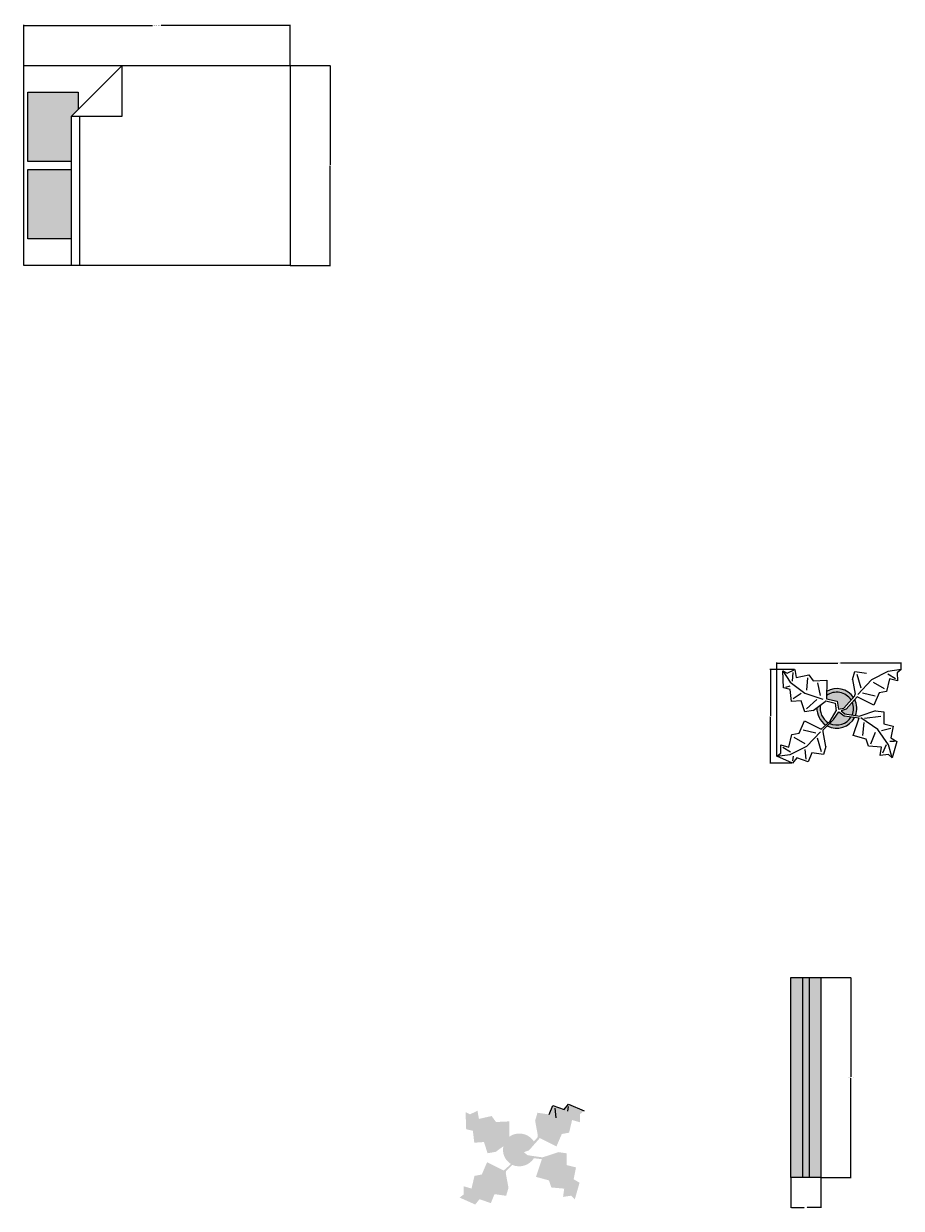
# Model space of a CAD drawing. Units: inches. Extents: x -494 to 1275, y 12 to 1194.
# Tile 6 of 8: x 704 to 968, y 781 to 1136. Entities that reach past the tile are written whole.
import ezdxf

# ---------------------------------------------------------------- set-up
doc = ezdxf.new("R2010")
doc.units = ezdxf.units.IN
doc.header["$MEASUREMENT"] = 0
for name, color, linetype, lineweight in [('A-ANNO-DIMS', 2, 'Continuous', 18), ('A-FURN', 8, 'Continuous', 18), ('A-GLAZ', 4, 'Continuous', 18), ('A-GLAZ-FRAM-PATT', 7, 'Continuous', 13), ('A-GLAZ-GLAS-PATT', 4, 'Continuous', 13), ('L-PLNT', 3, 'Continuous', 18)]:
    doc.layers.add(name, color=color, linetype=linetype, lineweight=lineweight)
doc.layers.add('A-FURN-PATT', color=254, linetype='Continuous', lineweight=13, true_color=0xfeeab9)
doc.layers.add('L-PLNT-PATT', color=114, linetype='Continuous', lineweight=13, true_color=0x139b48)
doc.styles.get("Standard").update_dxf_attribs({"font": 'arial.ttf'})
doc.dimstyles.get("Standard").update_dxf_attribs({"dimtxt": 0.18, "dimasz": 0.18, "dimexe": 0.18, "dimexo": 0.0625, "dimgap": 0.09, "dimtad": 0, "dimtih": 1, "dimtoh": 1, "dimdec": 4, "dimzin": 0, "dimdsep": 46, "dimlunit": 4, "dimtxsty": 'Standard', "dimcen": 0.09, "dimadec": 0, "dimazin": 0, "dimtfac": 1, "dimtdec": 4, "dimtofl": 0, "dimtmove": 0, "dimatfit": 3, "dimfxl": 1, "dimtolj": 1, "dimtzin": 0, "dimarcsym": 0})

# ---------------------------------------------------------------- blocks, each defined once
blk = doc.blocks.new('Bed - Queen')
for p, q in [((0, -80.00003), (0, 0)), ((0, 0), (59.99999, 0)), ((59.99999, 0), (59.99999, -80.00003)), ((7.99999, -1.2), (28.79998, -1.2)), ((7.99999, -14.4), (7.99999, -1.2)), ((28.79998, -1.2), (28.79998, -14.4)), ((31.19999, -1.2), (51.99999, -1.2)), ((31.19999, -14.4), (31.19999, -1.2)), ((51.99999, -1.2), (51.99999, -16.4)), ((0, -14.4), (44.8, -14.4)), ((44.8, -16.8), (0, -16.8)), ((59.99999, -29.6), (44.8, -14.4)), ((44.8, -14.4), (44.8, -29.6)), ((51.99999, -16.4), (46.79936, -16.4)), ((44.8, -29.6), (59.99999, -29.6)), ((59.99999, -80.00003), (0, -80.00003))]:
    blk.add_line(p, q)
blk = doc.blocks.new('WINDOW-60IN')
for p, q in [((3.5, 60), (3.5, 0)), ((5.5, 60), (5.5, 0))]:
    blk.add_line(p, q)
blk.add_lwpolyline([(9, 0), (0, 0), (0, 60), (9, 60)], close=True)
blk = doc.blocks.new('*D16')
at = {"layer": 'A-ANNO-DIMS', "color": 0, "lineweight": -2, "transparency": 16777216}
for p, q in [((704.14, 1123.82), (704.14, 1135.94)), ((704.32, 1135.76), (742.83, 1135.76)), ((783.96, 1135.76), (745.44, 1135.76)), ((784.14, 1123.82), (784.14, 1135.94))]:
    blk.add_line(p, q, dxfattribs=at)
at = {"layer": 'A-ANNO-DIMS', "color": 0, "transparency": 16777216}
for points in [[(704.32, 1135.79), (704.32, 1135.73), (704.14, 1135.76)], [(783.96, 1135.79), (783.96, 1135.73), (784.14, 1135.76)]]:
    blk.add_solid(points, dxfattribs=at)
at = {"layer": 'Defpoints', "color": 0, "transparency": 16777216}
for p in [(704.14, 1135.76), (704.14, 1123.76), (784.14, 1123.76)]:
    blk.add_point(p, dxfattribs=at)
at = {"layer": 'A-ANNO-DIMS', "color": 0, "transparency": 16777216, "insert": (744.14, 1135.76), "char_height": 0.18, "attachment_point": 5}
blk.add_mtext('\\A1;QUEEN BED 80 TYP.', dxfattribs=at)
blk = doc.blocks.new('*D17')
at = {"layer": 'A-ANNO-DIMS', "color": 0, "lineweight": -2, "transparency": 16777216}
for p, q in [((784.2, 1123.76), (796.32, 1123.76)), ((796.14, 1123.58), (796.14, 1093.94)), ((796.14, 1063.94), (796.14, 1093.58)), ((784.2, 1063.76), (796.32, 1063.76))]:
    blk.add_line(p, q, dxfattribs=at)
at = {"layer": 'A-ANNO-DIMS', "color": 0, "transparency": 16777216}
for points in [[(796.11, 1123.58), (796.17, 1123.58), (796.14, 1123.76)], [(796.11, 1063.94), (796.17, 1063.94), (796.14, 1063.76)]]:
    blk.add_solid(points, dxfattribs=at)
at = {"layer": 'Defpoints', "color": 0, "transparency": 16777216}
for p in [(784.14, 1123.76), (796.14, 1123.76), (784.14, 1063.76)]:
    blk.add_point(p, dxfattribs=at)
at = {"layer": 'A-ANNO-DIMS', "color": 0, "transparency": 16777216, "insert": (796.14, 1093.76), "char_height": 0.18, "attachment_point": 5}
blk.add_mtext('\\A1;60 TYP.', dxfattribs=at)
blk = doc.blocks.new('*D20')
at = {"layer": 'A-ANNO-DIMS', "color": 0, "lineweight": -2, "transparency": 16777216}
for p, q in [((943.57, 849.92), (952.69, 849.92)), ((952.51, 849.74), (952.51, 820.1)), ((952.51, 790.1), (952.51, 819.73)), ((943.57, 789.92), (952.69, 789.92))]:
    blk.add_line(p, q, dxfattribs=at)
at = {"layer": 'A-ANNO-DIMS', "color": 0, "transparency": 16777216}
for points in [[(952.48, 849.74), (952.54, 849.74), (952.51, 849.92)], [(952.48, 790.1), (952.54, 790.1), (952.51, 789.92)]]:
    blk.add_solid(points, dxfattribs=at)
at = {"layer": 'Defpoints', "color": 0, "transparency": 16777216}
for p in [(943.51, 849.92), (952.51, 849.92), (943.51, 789.92)]:
    blk.add_point(p, dxfattribs=at)
at = {"layer": 'A-ANNO-DIMS', "color": 0, "transparency": 16777216, "insert": (952.51, 819.92), "char_height": 0.18, "attachment_point": 5}
blk.add_mtext('\\A1;WINDOW A 60 TYP.', dxfattribs=at)
blk = doc.blocks.new('*D21')
at = {"layer": 'A-ANNO-DIMS', "color": 0, "lineweight": -2, "transparency": 16777216}
for p, q in [((934.51, 789.85), (934.51, 780.74)), ((943.51, 789.85), (943.51, 780.74)), ((934.69, 780.92), (938.55, 780.92)), ((943.33, 780.92), (939.46, 780.92))]:
    blk.add_line(p, q, dxfattribs=at)
at = {"layer": 'A-ANNO-DIMS', "color": 0, "transparency": 16777216}
for points in [[(934.69, 780.95), (934.69, 780.89), (934.51, 780.92)], [(943.33, 780.95), (943.33, 780.89), (943.51, 780.92)]]:
    blk.add_solid(points, dxfattribs=at)
at = {"layer": 'Defpoints', "color": 0, "transparency": 16777216}
for p in [(934.51, 789.92), (943.51, 789.92), (943.51, 780.92)]:
    blk.add_point(p, dxfattribs=at)
at = {"layer": 'A-ANNO-DIMS', "color": 0, "transparency": 16777216, "insert": (939.01, 780.92), "char_height": 0.18, "attachment_point": 5}
blk.add_mtext('\\A1;9 TYP.', dxfattribs=at)
blk = doc.blocks.new('*D71')
at = {"layer": 'A-ANNO-DIMS', "color": 0, "lineweight": -2, "transparency": 16777216}
for p, q in [((930.32, 916.44), (930.32, 944.55)), ((930.5, 944.37), (948.63, 944.37)), ((967.54, 944.37), (949.41, 944.37)), ((967.72, 942.44), (967.72, 944.55))]:
    blk.add_line(p, q, dxfattribs=at)
at = {"layer": 'A-ANNO-DIMS', "color": 0, "transparency": 16777216}
for points in [[(930.5, 944.4), (930.5, 944.34), (930.32, 944.37)], [(967.54, 944.4), (967.54, 944.34), (967.72, 944.37)]]:
    blk.add_solid(points, dxfattribs=at)
at = {"layer": 'Defpoints', "color": 0, "transparency": 16777216}
for p in [(967.72, 944.37), (967.72, 942.37), (930.32, 916.38)]:
    blk.add_point(p, dxfattribs=at)
at = {"layer": 'A-ANNO-DIMS', "color": 0, "transparency": 16777216, "insert": (949.02, 944.37), "char_height": 0.18, "attachment_point": 5}
blk.add_mtext('\\A1;37.39', dxfattribs=at)
blk = doc.blocks.new('*D72')
at = {"layer": 'A-ANNO-DIMS', "color": 0, "lineweight": -2, "transparency": 16777216}
for p, q in [((935.65, 942.46), (928.23, 942.46)), ((928.41, 942.28), (928.41, 928.56)), ((928.41, 914.47), (928.41, 928.19)), ((934.97, 914.29), (928.23, 914.29))]:
    blk.add_line(p, q, dxfattribs=at)
at = {"layer": 'A-ANNO-DIMS', "color": 0, "transparency": 16777216}
for points in [[(928.38, 942.28), (928.44, 942.28), (928.41, 942.46)], [(928.38, 914.47), (928.44, 914.47), (928.41, 914.29)]]:
    blk.add_solid(points, dxfattribs=at)
at = {"layer": 'Defpoints', "color": 0, "transparency": 16777216}
for p in [(928.41, 942.46), (935.71, 942.46), (935.03, 914.29)]:
    blk.add_point(p, dxfattribs=at)
at = {"layer": 'A-ANNO-DIMS', "color": 0, "transparency": 16777216, "insert": (928.41, 928.38), "char_height": 0.18, "attachment_point": 5}
blk.add_mtext('\\A1;28.165', dxfattribs=at)

msp = doc.modelspace()

# ---------------------------------------------------------------- hatches: boundary and pattern name
at = {"layer": 'A-FURN-PATT'}
h = msp.add_hatch(color=256, dxfattribs=at)
h.dxf.hatch_style = 1
h.paths.add_polyline_path([(705.3369, 1094.9575), (718.5369, 1094.9575), (718.5369, 1108.5575), (720.5369, 1110.5575), (720.5369, 1115.7575), (705.3369, 1115.7575)])
h.paths.add_polyline_path([(705.3369, 1071.7575), (718.5369, 1071.7575), (718.5369, 1092.5575), (705.3369, 1092.5575)])
at = {"layer": 'A-GLAZ-FRAM-PATT'}
h = msp.add_hatch(color=256, dxfattribs=at)
h.dxf.hatch_style = 1
h.paths.add_polyline_path([(940.0053, 789.9155), (943.5053, 789.9155), (943.5053, 849.9155), (940.0053, 849.9155)])
h.paths.add_polyline_path([(938.0053, 849.9155), (934.5053, 849.9155), (934.5053, 789.9155), (938.0053, 789.9155)])
at = {"layer": 'A-GLAZ-GLAS-PATT'}
h = msp.add_hatch(color=256, dxfattribs=at)
h.dxf.hatch_style = 1
h.paths.add_polyline_path([(940.0053, 849.9155), (938.0053, 849.9155), (938.0053, 789.9155), (940.0053, 789.9155)])
at = {"layer": 'L-PLNT-PATT'}
h = msp.add_hatch(color=256, dxfattribs=at)
h.dxf.hatch_style = 1
h.paths.add_polyline_path([(944.9959, 925.7613), (945.7664, 926.4537, -0.3202719), (943.4786, 931.7921), (942.3823, 930.9828, 0.26249769)])
h.paths.add_polyline_path([(945.2783, 935.8722), (945.2615, 933.6641), (948.4121, 932.8763), (948.819, 930.529), (950.4465, 930.7898), (953.3756, 934.0403, 0.39031988)])
h = msp.add_hatch(color=256, dxfattribs=at)
h.dxf.hatch_style = 1
h.paths.add_polyline_path([(951.1586, 930.529), (949.6327, 930.0073), (950.7517, 929.0945), (952.965, 928.7721, 0.19674885), (952.9711, 932.5841)])
h.paths.add_polyline_path([(953.9663, 928.6262, 0.21301293), (953.7156, 933.4282), (952.9711, 932.5841, -0.19674885), (952.965, 928.7721)])
h.paths.add_polyline_path([(953.7342, 928.0648), (950.5771, 928.4684), (948.9207, 929.7465), (947.3949, 927.3992), (945.4776, 925.4839, 0.41243311)])
h = msp.add_hatch(color=256, dxfattribs=at)
h.dxf.hatch_style = 1
h.paths.add_polyline_path([(850.0221, 806.7469), (845.9956, 806.5538), (844.6676, 808.3528), (840.8596, 807.4873), (840.431, 809.9503), (838.1866, 808.8492), (836.85, 809.5302), (837.0346, 804.3857), (839.0436, 803.9232), (839.4637, 800.3422), (842.3721, 800.5438), (843.4647, 797.1813), (845.9277, 797.6098), (849.5257, 800.2659), (849.7494, 800.4883), (852.5199, 799.8475), (852.825, 797.5001), (851.0315, 794.438), (848.3241, 792.0049), (843.3184, 794.4935), (841.7268, 790.7899), (839.5277, 790.3849), (838.6364, 786.5829), (836.2348, 787.2774), (836.2404, 784.7774), (835.0425, 783.8747), (839.7473, 781.7854), (841.0436, 783.3883), (844.4463, 782.196), (845.5402, 784.8985), (849.0413, 784.4065), (849.7359, 786.8081), (848.9259, 791.2062), (848.9926, 791.7747), (852.113, 794.892), (853.6388, 797.2393), (855.2952, 795.9612), (859.7613, 795.3902), (857.9935, 790.0869), (861.8826, 789.0262), (862.5897, 786.9049), (866.4788, 786.5513), (866.1253, 784.0765), (868.6001, 784.43), (869.6608, 783.3694), (871.075, 788.3191), (869.3072, 789.3798), (870.0143, 792.9153), (867.1859, 793.6224), (867.1859, 797.158), (864.711, 797.5115), (859.9455, 795.9353), (855.4698, 796.5873), (854.3508, 797.5001), (855.8767, 798.0218), (859.1537, 801.7372), (864.1594, 799.2486), (865.751, 802.9522), (867.95, 803.3572), (868.8414, 807.1593), (871.243, 806.4647), (871.2373, 808.9647), (872.4353, 809.8674), (867.7305, 811.9567), (866.4342, 810.3538), (863.0314, 811.5461), (861.9376, 808.8436), (858.4364, 809.3356), (857.7419, 806.934), (858.5519, 802.5359), (858.4851, 801.9674), (855.1646, 798.2826), (853.5371, 798.0218), (853.1302, 800.3691), (849.9796, 801.1569)])
h.paths.add_polyline_path([(849.9872, 802.1467), (849.9796, 801.1569), (853.1302, 800.3691), (853.5371, 798.0218), (855.1646, 798.2826), (857.3713, 800.7314, 0.42214063)], flags=17)
h.paths.add_polyline_path([(852.825, 797.5001), (852.5199, 799.8475), (849.7494, 800.4883), (849.5257, 800.2659), (848.1961, 799.2843, 0.3201537), (850.4845, 793.9464), (851.0315, 794.438)], flags=17)
h.paths.add_polyline_path([(857.3957, 795.6926), (855.2952, 795.9612), (853.6388, 797.2393), (852.113, 794.892), (850.8876, 793.6677, 0.36518483)], flags=17)

# ---------------------------------------------------------------- linework, layer by layer
at = {"layer": 'L-PLNT'}
for p, q in [((932.1319, 942.0374), (934.3425, 938.6664)), ((932.1319, 942.0374), (933.4685, 941.3564)), ((932.3165, 936.8929), (932.1319, 942.0374)), ((933.4685, 941.3564), (935.7129, 942.4575)), ((935.015, 938.885), (935.2589, 941.5665)), ((935.7129, 942.4575), (936.1415, 939.9945)), ((936.1415, 939.9945), (939.9495, 940.86)), ((939.4955, 939.969), (939.243, 936.1695)), ((939.9495, 940.86), (941.2775, 939.061)), ((941.2775, 939.061), (945.304, 939.2541)), ((945.304, 939.2541), (945.2615, 933.6641)), ((953.0238, 939.4412), (953.7183, 941.8428)), ((953.0238, 939.4412), (953.8338, 935.0431)), ((953.7183, 941.8428), (957.2195, 941.3508)), ((954.3202, 941.0442), (955.5295, 936.9469)), ((958.724, 939.3542), (954.6171, 934.9628)), ((963.7183, 941.8655), (958.724, 939.3542)), ((964.1233, 939.6665), (963.2319, 935.8644)), ((963.6199, 941.1653), (965.9231, 939.7705)), ((967.7172, 942.3746), (963.7183, 941.8655)), ((966.5249, 938.9719), (964.1233, 939.6665)), ((967.7172, 942.3746), (966.5192, 941.4719)), ((966.5192, 941.4719), (966.5249, 938.9719)), ((934.3255, 936.4304), (932.3165, 936.8929)), ((932.989, 937.1114), (934.334, 937.5484)), ((934.7456, 932.8494), (934.3255, 936.4304)), ((934.3425, 938.6664), (938.789, 935.2785)), ((943.4795, 934.572), (942.614, 938.38)), ((956.0329, 935.4481), (959.8349, 934.5567)), ((962.6301, 936.6631), (959.3258, 938.5556)), ((961.0329, 935.4594), (959.4413, 931.7558)), ((963.2319, 935.8644), (961.0329, 935.4594)), ((937.654, 933.051), (934.7456, 932.8494)), ((935.1995, 933.7404), (937.671, 935.287)), ((938.7466, 929.6885), (937.654, 933.051)), ((938.789, 935.2785), (944.1407, 933.5488)), ((939.2006, 930.5795), (942.3531, 933.4625)), ((941.2096, 930.117), (944.8076, 932.7731)), ((944.8076, 932.7731), (945.0313, 932.9955)), ((945.0313, 932.9955), (947.8018, 932.3547)), ((945.2615, 933.6641), (948.4121, 932.8763)), ((947.8018, 932.3547), (948.1069, 930.0073)), ((947.8018, 932.3547), (947.8018, 932.3547)), ((948.4121, 932.8763), (948.819, 930.529)), ((950.4465, 930.7898), (953.767, 934.4746)), ((954.4356, 934.2444), (951.1586, 930.529)), ((953.767, 934.4746), (953.8338, 935.0431)), ((959.4413, 931.7558), (954.4356, 934.2444)), ((941.2096, 930.117), (938.7466, 929.6885)), ((946.3134, 926.9452), (948.1069, 930.0073)), ((947.3949, 927.3992), (948.9207, 929.7465)), ((948.819, 930.529), (950.4465, 930.7898)), ((948.9207, 929.7465), (950.5771, 928.4684)), ((951.1586, 930.529), (949.6327, 930.0073)), ((949.6327, 930.0073), (950.7517, 929.0945)), ((950.5771, 928.4684), (955.0432, 927.8974)), ((950.7517, 929.0945), (955.2274, 928.4425)), ((959.9929, 930.0187), (955.2274, 928.4425)), ((956.6868, 927.8147), (961.5297, 928.3896)), ((959.9929, 930.0187), (962.4678, 929.6652)), ((962.4678, 929.6652), (962.4678, 926.1296)), ((937.0087, 923.2971), (938.6003, 927.0007)), ((938.6003, 927.0007), (943.606, 924.5121)), ((946.3134, 926.9452), (943.606, 924.5121)), ((944.2745, 924.2819), (947.3949, 927.3992)), ((953.2754, 922.5941), (955.0432, 927.8974)), ((960.7001, 924.3619), (955.5514, 927.8828)), ((956.4574, 926.4832), (956.1039, 922.5941)), ((962.4678, 926.1296), (965.2962, 925.4225)), ((965.2962, 925.4225), (964.5891, 921.887)), ((933.9183, 919.0901), (934.8096, 922.8921)), ((934.8096, 922.8921), (937.0087, 923.2971)), ((935.4114, 922.0935), (938.7158, 920.201)), ((942.0087, 923.3084), (938.2067, 924.1998)), ((939.3176, 919.4023), (943.4277, 923.7478)), ((943.7214, 917.7123), (942.5121, 921.8096)), ((944.2078, 923.7134), (944.2745, 924.2819)), ((945.0178, 919.3153), (944.2078, 923.7134)), ((957.1645, 921.5334), (953.2754, 922.5941)), ((957.8716, 919.4121), (957.1645, 921.5334)), ((958.5787, 920.1192), (959.9929, 923.6547)), ((963.882, 919.7657), (960.7001, 924.3619)), ((964.5891, 924.7154), (961.7607, 924.0083)), ((964.5891, 921.887), (966.3569, 920.8263)), ((931.5167, 919.7846), (933.9183, 919.0901)), ((931.5223, 917.2846), (931.5167, 919.7846)), ((934.4217, 917.5912), (932.1185, 918.986)), ((934.3233, 916.891), (939.3176, 919.4023)), ((939.1264, 915.5019), (938.8198, 918.4012)), ((945.0178, 919.3153), (944.3232, 916.9137)), ((961.7607, 919.0585), (957.8716, 919.4121)), ((961.4072, 916.5837), (961.7607, 919.0585)), ((963.1749, 919.7657), (962.1143, 917.2908)), ((964.9427, 915.8766), (963.882, 919.7657)), ((965.6498, 920.8263), (964.2356, 920.8263)), ((966.3569, 920.8263), (964.9427, 915.8766)), ((930.3244, 916.3819), (931.5223, 917.2846)), ((930.3244, 916.3819), (934.3233, 916.891)), ((935.0292, 914.2926), (930.3244, 916.3819)), ((936.3255, 915.8955), (935.0292, 914.2926)), ((935.1276, 914.9928), (935.3244, 916.3932)), ((939.7282, 914.7032), (936.3255, 915.8955)), ((940.8221, 917.4057), (939.7282, 914.7032)), ((944.3232, 916.9137), (940.8221, 917.4057)), ((963.882, 916.9372), (961.4072, 916.5837)), ((964.9427, 915.8766), (963.882, 916.9372)), ((861.9376, 808.8436), (863.0314, 811.5461)), ((863.0314, 811.5461), (866.4342, 810.3538)), ((866.4342, 810.3538), (867.7305, 811.9567)), ((867.6321, 811.2565), (867.4353, 809.8561)), ((867.7305, 811.9567), (872.4353, 809.8674)), ((863.6333, 810.7474), (863.9398, 807.8481))]:
    msp.add_line(p, q, dxfattribs=at)
for centre, radius, start, end in [((948.3324, 930.56), 6.1275, 34.37569, 120.1028), ((948.2723, 930.3525), 5.2461, 33.82192, 124.9414), ((948.3119, 930.6855), 5.0312, 337.646935, 22.16977), ((948.461, 930.7463), 5.8995, 338.938822, 27.038882), ((948.3193, 930.6897), 5.9443, 177.174105, 236.006825), ((948.3621, 930.7255), 4.9986, 167.68042, 238.677422), ((948.3076, 930.9278), 6.1356, 242.529166, 332.184156), ((948.2222, 931.0486), 5.2883, 247.3711, 327.472)]:
    msp.add_arc(centre, radius, start, end, dxfattribs=at)

# ---------------------------------------------------------------- block references
at = {"layer": 'A-FURN', "rotation": 90}
msp.add_blockref('Bed - Queen', (704.1369, 1063.7575), dxfattribs=at)
at = {"layer": 'A-GLAZ'}
msp.add_blockref('WINDOW-60IN', (934.505, 789.916), dxfattribs=at)

# ---------------------------------------------------------------- dimensions: what is measured, and where the dimension line sits
at = {"layer": 'A-ANNO-DIMS'}
for base, p1, p2, angle, text, picture, middle in [((704.1369, 1135.7575), (784.1369, 1123.7575), (704.1369, 1123.7575), 180, 'QUEEN BED <> TYP.', '*D16', (744.1369, 1135.7575)), ((796.1369, 1123.7575), (784.1369, 1063.7575), (784.1369, 1123.7575), 90, '<> TYP.', '*D17', (796.1369, 1093.7575)), ((952.5053, 849.9155), (943.5053, 789.9155), (943.5053, 849.9155), 90, 'WINDOW A <> TYP.', '*D20', (952.5053, 819.9155))]:
    dim = msp.add_linear_dim(base=base, p1=p1, p2=p2, angle=angle, text=text, dimstyle='Standard', override={"dimdec": 0, "dimlfac": 1, "dimrnd": 0, "dimzin": 0, "dimdsep": 46, "dimlunit": 2}, dxfattribs=at)
    dim.commit()
    dim.dimension.update_dxf_attribs({"geometry": picture, "text_midpoint": middle})
dim = msp.add_linear_dim(base=(967.7172, 944.3675), p1=(930.3244, 916.3819), p2=(967.7172, 942.3746), dimstyle='Standard', override={"dimdec": 2, "dimlfac": 1, "dimrnd": 0, "dimzin": 0, "dimdsep": 46, "dimlunit": 2}, dxfattribs=at)
dim.commit()
dim.dimension.update_dxf_attribs({"geometry": '*D71', "text_midpoint": (949.0208, 944.3675)})
dim = msp.add_linear_dim(base=(928.4144, 942.4575), p1=(935.0292, 914.2926), p2=(935.7129, 942.4575), angle=90, dimstyle='Standard', override={"dimdec": 3, "dimlfac": 1, "dimrnd": 0, "dimzin": 0, "dimdsep": 46, "dimlunit": 2}, dxfattribs=at)
dim.commit()
dim.dimension.update_dxf_attribs({"geometry": '*D72', "text_midpoint": (928.4144, 928.3751)})
dim = msp.add_linear_dim(base=(943.5053, 780.9155), p1=(934.5053, 789.9155), p2=(943.5053, 789.9155), text='<> TYP.', dimstyle='Standard', override={"dimdec": 0, "dimlfac": 1, "dimrnd": 0, "dimzin": 0, "dimdsep": 46, "dimlunit": 2}, dxfattribs=at)
dim.commit()
dim.dimension.update_dxf_attribs({"geometry": '*D21', "text_midpoint": (939.0053, 780.9155)})

doc.saveas('drawing.dxf')
